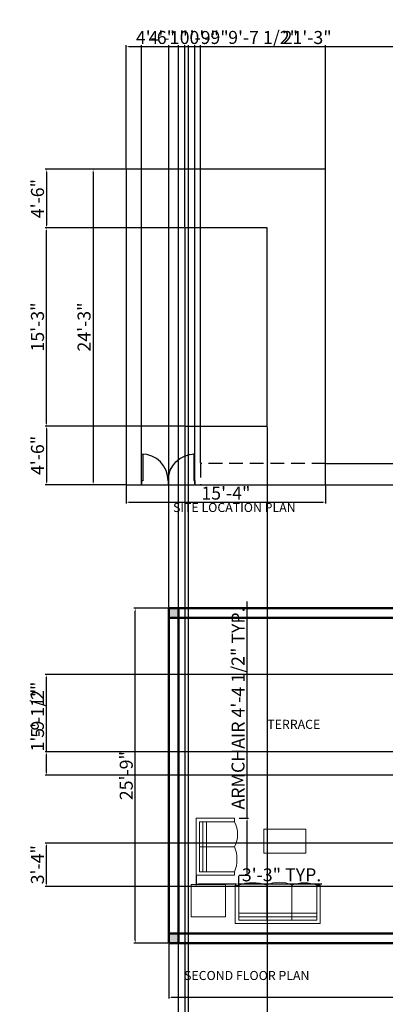
# Model space of a CAD drawing. Units: inches. Extents: x 1367 to 2309, y 1406 to 3826.
# Tile 7 of 9: x 1367 to 1704, y 2918 to 3826. Entities that reach past the tile are written whole.
import ezdxf

# ---------------------------------------------------------------- set-up
doc = ezdxf.new("R2010")
doc.units = ezdxf.units.IN
doc.linetypes.add('DASHED', pattern=[19.05, 12.7, -6.35])
for name, color, linetype, lineweight in [('A-ANNO-DIMS', 2, 'Continuous', 18), ('A-ANNO-TEXT', 7, 'Continuous', 25), ('A-AREA-IDEN', 3, 'Continuous', 18), ('A-DOOR', 4, 'Continuous', 25), ('A-FURN', 8, 'Continuous', 18), ('A-WALL', 7, 'Continuous', 50), ('A-WALL-PATT', 8, 'Continuous', 18), ('C-PROP', 7, 'Continuous', 25), ('C-PROP-LINE', 1, 'DASHED', 25)]:
    doc.layers.add(name, color=color, linetype=linetype, lineweight=lineweight)
doc.styles.get("Standard").update_dxf_attribs({"font": 'arial.ttf'})
doc.dimstyles.new('ISO-25', dxfattribs={"dimtxt": 12, "dimasz": 2.5, "dimexe": 1.25, "dimexo": 0.625, "dimtad": 1, "dimdec": 0, "dimlunit": 4, "dimtxsty": 'Standard', "dimcen": 2.5, "dimadec": 0, "dimazin": 0, "dimtfac": 1, "dimtdec": 0, "dimtmove": 0, "dimatfit": 3, "dimfxl": 1, "dimarcsym": 0})

# ---------------------------------------------------------------- blocks, each defined once
blk = doc.blocks.new('*U2')
for p, q in [((0, 0), (0, -6)), ((40, 0), (40, -6))]:
    blk.add_line(p, q)
blk.add_lwpolyline([(0, 0), (0, 40), (1.75, 40), (1.75, 0)], close=True)
blk.add_arc((0, 0), 40, 0, 90)
blk = doc.blocks.new('*D38')
at = {"layer": 'A-ANNO-DIMS', "color": 0, "lineweight": -2, "transparency": 16777216}
for p, q in [((1503.75, 3283.62), (1472.13, 3283.62)), ((1473.38, 2977.12), (1473.38, 3281.12)), ((1503.75, 2974.62), (1472.13, 2974.62))]:
    blk.add_line(p, q, dxfattribs=at)
at = {"layer": 'A-ANNO-DIMS', "color": 0, "lineweight": 100, "transparency": 16777216}
for points in [[(1472.96, 3281.12), (1473.79, 3281.12), (1473.38, 3283.62)], [(1472.96, 2977.12), (1473.79, 2977.12), (1473.38, 2974.62)]]:
    blk.add_solid(points, dxfattribs=at)
at = {"layer": 'Defpoints', "color": 0, "lineweight": 100, "transparency": 16777216}
for p in [(1473.38, 3283.62), (1504.37, 3283.62), (1504.37, 2974.62)]:
    blk.add_point(p, dxfattribs=at)
at = {"layer": 'A-ANNO-DIMS', "color": 0, "transparency": 16777216, "insert": (1466.62, 3129.12), "char_height": 12, "attachment_point": 5, "rotation": 90}
blk.add_mtext('25\'-9"', dxfattribs=at)
blk = doc.blocks.new('*D39')
at = {"layer": 'A-ANNO-DIMS', "color": 0, "lineweight": -2, "transparency": 16777216}
for p, q in [((1504.37, 2973.99), (1504.37, 2923.6)), ((2113.4, 2973.99), (2113.4, 2923.6)), ((1506.87, 2924.85), (2110.9, 2924.85))]:
    blk.add_line(p, q, dxfattribs=at)
at = {"layer": 'A-ANNO-DIMS', "color": 0, "lineweight": 100, "transparency": 16777216}
for points in [[(1506.87, 2925.27), (1506.87, 2924.44), (1504.37, 2924.85)], [(2110.9, 2925.27), (2110.9, 2924.44), (2113.4, 2924.85)]]:
    blk.add_solid(points, dxfattribs=at)
at = {"layer": 'Defpoints', "color": 0, "lineweight": 100, "transparency": 16777216}
for p in [(1504.37, 2974.62), (2113.4, 2974.62), (2113.4, 2924.85)]:
    blk.add_point(p, dxfattribs=at)
at = {"layer": 'A-ANNO-DIMS', "color": 0, "transparency": 16777216, "insert": (1808.89, 2931.6), "char_height": 12, "attachment_point": 5}
blk.add_mtext('50\'-9"', dxfattribs=at)
blk = doc.blocks.new('*D40')
at = {"layer": 'A-ANNO-DIMS', "color": 0, "lineweight": -2, "transparency": 16777216}
for p, q in [((1464.39, 3688.12), (1433.26, 3688.12)), ((1434.51, 3685.62), (1434.51, 3399.83)), ((1464.39, 3397.33), (1433.26, 3397.33))]:
    blk.add_line(p, q, dxfattribs=at)
at = {"layer": 'A-ANNO-DIMS', "color": 0, "lineweight": 100, "transparency": 16777216}
for points in [[(1434.09, 3685.62), (1434.92, 3685.62), (1434.51, 3688.12)], [(1434.09, 3399.83), (1434.92, 3399.83), (1434.51, 3397.33)]]:
    blk.add_solid(points, dxfattribs=at)
at = {"layer": 'Defpoints', "color": 0, "lineweight": 100, "transparency": 16777216}
for p in [(1465.02, 3688.12), (1434.51, 3397.33), (1465.02, 3397.33)]:
    blk.add_point(p, dxfattribs=at)
at = {"layer": 'A-ANNO-DIMS', "color": 0, "transparency": 16777216, "insert": (1427.75, 3542.73), "char_height": 12, "attachment_point": 5, "rotation": 90}
blk.add_mtext('24\'-3"', dxfattribs=at)
blk = doc.blocks.new('*D41')
at = {"layer": 'A-ANNO-DIMS', "color": 0, "lineweight": -2, "transparency": 16777216}
for p, q in [((1465.02, 3396.71), (1465.02, 3380.03)), ((1648.94, 3396.71), (1648.94, 3380.03)), ((1467.52, 3381.28), (1646.44, 3381.28))]:
    blk.add_line(p, q, dxfattribs=at)
at = {"layer": 'A-ANNO-DIMS', "color": 0, "lineweight": 100, "transparency": 16777216}
for points in [[(1467.52, 3381.7), (1467.52, 3380.86), (1465.02, 3381.28)], [(1646.44, 3381.7), (1646.44, 3380.86), (1648.94, 3381.28)]]:
    blk.add_solid(points, dxfattribs=at)
at = {"layer": 'Defpoints', "color": 0, "lineweight": 100, "transparency": 16777216}
for p in [(1465.02, 3397.33), (1648.94, 3397.33), (1648.94, 3381.28)]:
    blk.add_point(p, dxfattribs=at)
at = {"layer": 'A-ANNO-DIMS', "color": 0, "transparency": 16777216, "insert": (1556.98, 3388.03), "char_height": 12, "attachment_point": 5}
blk.add_mtext('15\'-4"', dxfattribs=at)
blk = doc.blocks.new('SOFA-3')
for p, q in [((3.39, 35.52), (0, 35.52)), ((0, 35.52), (0, 0)), ((29.28, 35.52), (29.28, 3.13)), ((52.37, 35.52), (52.37, 3.13)), ((75.45, 35.52), (78.61, 35.52)), ((78.61, 0), (78.61, 35.52)), ((0, 0), (78.61, 0))]:
    blk.add_line(p, q)
blk.add_lwpolyline([(3.39, 35.52), (3.39, 3.13), (75.45, 3.13), (75.45, 35.52)])
for centre, radius, start, end in [((16.33, -1.36), 39.09, 70.66096, 109.33904), ((40.82, 12.11), 26.1, 63.74962, 116.25038), ((63.91, 5.49), 32.17, 68.97185, 111.02815)]:
    blk.add_arc(centre, radius, start, end)
blk = doc.blocks.new('ARMCHAIR')
for p, q in [((0, 52.73), (0, 0)), ((35.52, 52.73), (0, 52.73)), ((35.52, 49.34), (3.13, 49.34)), ((35.52, 49.34), (35.52, 52.73)), ((35.52, 26.25), (3.13, 26.25)), ((35.52, 3.16), (35.52, 0)), ((0, 0), (35.52, 0))]:
    blk.add_line(p, q)
blk.add_lwpolyline([(3.13, 49.34), (3.13, 3.16), (35.52, 3.16)])
for centre, radius, start, end in [((12.11, 37.79), 26.1, 333.74962, 26.25038), ((5.49, 14.7), 32.17, 338.97185, 21.02815)]:
    blk.add_arc(centre, radius, start, end)
blk = doc.blocks.new('*D53')
at = {"layer": 'A-ANNO-DIMS', "color": 0, "lineweight": -2, "transparency": 16777216}
for p, q in [((1576.53, 3089.97), (1576.53, 3289.6)), ((1569.25, 3089.97), (1577.78, 3089.97)), ((1576.53, 3039.74), (1576.53, 3087.47)), ((1569.25, 3037.24), (1577.78, 3037.24))]:
    blk.add_line(p, q, dxfattribs=at)
at = {"layer": 'A-ANNO-DIMS', "color": 0, "lineweight": 100, "transparency": 16777216}
for points in [[(1576.11, 3087.47), (1576.95, 3087.47), (1576.53, 3089.97)], [(1576.11, 3039.74), (1576.95, 3039.74), (1576.53, 3037.24)]]:
    blk.add_solid(points, dxfattribs=at)
at = {"layer": 'Defpoints', "color": 0, "lineweight": 100, "transparency": 16777216}
for p in [(1568.62, 3089.97), (1576.53, 3089.97), (1568.62, 3037.24)]:
    blk.add_point(p, dxfattribs=at)
at = {"layer": 'A-ANNO-DIMS', "color": 0, "transparency": 16777216, "insert": (1569.7, 3191.04), "char_height": 12, "attachment_point": 5, "rotation": 90}
blk.add_mtext('ARMCHAIR 4\'-4 1/2" TYP.', dxfattribs=at)
blk = doc.blocks.new('*D54')
at = {"layer": 'A-ANNO-DIMS', "color": 0, "lineweight": -2, "transparency": 16777216}
for p, q in [((1529.51, 3036.62), (1529.51, 3028.08)), ((1568.62, 3036.62), (1568.62, 3028.08)), ((1532.01, 3029.33), (1566.12, 3029.33)), ((1568.62, 3029.33), (1645.51, 3029.33))]:
    blk.add_line(p, q, dxfattribs=at)
at = {"layer": 'A-ANNO-DIMS', "color": 0, "lineweight": 100, "transparency": 16777216}
for points in [[(1532.01, 3029.75), (1532.01, 3028.92), (1529.51, 3029.33)], [(1566.12, 3029.75), (1566.12, 3028.92), (1568.62, 3029.33)]]:
    blk.add_solid(points, dxfattribs=at)
at = {"layer": 'Defpoints', "color": 0, "lineweight": 100, "transparency": 16777216}
for p in [(1529.51, 3037.24), (1568.62, 3037.24), (1568.62, 3029.33)]:
    blk.add_point(p, dxfattribs=at)
at = {"layer": 'A-ANNO-DIMS', "color": 0, "transparency": 16777216, "insert": (1608.31, 3036.09), "char_height": 12, "attachment_point": 5}
blk.add_mtext('3\'-3" TYP.', dxfattribs=at)
blk = doc.blocks.new('*D87')
at = {"layer": 'A-ANNO-DIMS', "color": 0, "lineweight": -2, "transparency": 16777216}
for p, q in [((1513.37, 2814.79), (1513.37, 3802.6)), ((1515.87, 3801.35), (2110.9, 3801.35)), ((2113.4, 2814.79), (2113.4, 3802.6))]:
    blk.add_line(p, q, dxfattribs=at)
at = {"layer": 'A-ANNO-DIMS', "color": 0, "lineweight": 100, "transparency": 16777216}
for points in [[(1515.87, 3801.77), (1515.87, 3800.93), (1513.37, 3801.35)], [(2110.9, 3801.77), (2110.9, 3800.93), (2113.4, 3801.35)]]:
    blk.add_solid(points, dxfattribs=at)
at = {"layer": 'Defpoints', "color": 0, "lineweight": 100, "transparency": 16777216}
for p in [(2113.4, 3801.35), (1513.37, 2814.17), (2113.4, 2814.17)]:
    blk.add_point(p, dxfattribs=at)
at = {"layer": 'A-ANNO-DIMS', "color": 0, "transparency": 16777216, "insert": (1813.39, 3808.1), "char_height": 12, "attachment_point": 5}
blk.add_mtext('50\'-0"', dxfattribs=at)
blk = doc.blocks.new('*D88')
at = {"layer": 'A-ANNO-DIMS', "color": 0, "lineweight": -2, "transparency": 16777216}
for p, q in [((1513.37, 2814.79), (1513.37, 3802.6)), ((1515.87, 3801.35), (1519.87, 3801.35)), ((1522.37, 2805.79), (1522.37, 3802.6)), ((1522.37, 3801.35), (1558.02, 3801.35))]:
    blk.add_line(p, q, dxfattribs=at)
at = {"layer": 'A-ANNO-DIMS', "color": 0, "lineweight": 100, "transparency": 16777216}
for points in [[(1515.87, 3801.77), (1515.87, 3800.93), (1513.37, 3801.35)], [(1519.87, 3801.77), (1519.87, 3800.93), (1522.37, 3801.35)]]:
    blk.add_solid(points, dxfattribs=at)
at = {"layer": 'Defpoints', "color": 0, "lineweight": 100, "transparency": 16777216}
for p in [(1522.37, 3801.35), (1513.37, 2814.17), (1522.37, 2805.17)]:
    blk.add_point(p, dxfattribs=at)
at = {"layer": 'A-ANNO-DIMS', "color": 0, "transparency": 16777216, "insert": (1541.44, 3808.1), "char_height": 12, "attachment_point": 5}
blk.add_mtext('0\'-9"', dxfattribs=at)
blk = doc.blocks.new('*D103')
at = {"layer": 'A-ANNO-DIMS', "color": 0, "lineweight": -2, "transparency": 16777216}
for p, q in [((1504.37, 3284.24), (1504.37, 3802.6)), ((1506.87, 3801.35), (1756.92, 3801.35)), ((1759.42, 3284.24), (1759.42, 3802.6))]:
    blk.add_line(p, q, dxfattribs=at)
at = {"layer": 'A-ANNO-DIMS', "color": 0, "lineweight": 100, "transparency": 16777216}
for points in [[(1506.87, 3801.77), (1506.87, 3800.93), (1504.37, 3801.35)], [(1756.92, 3801.77), (1756.92, 3800.93), (1759.42, 3801.35)]]:
    blk.add_solid(points, dxfattribs=at)
at = {"layer": 'Defpoints', "color": 0, "lineweight": 100, "transparency": 16777216}
for p in [(1759.42, 3801.35), (1504.37, 3283.62), (1759.42, 3283.62)]:
    blk.add_point(p, dxfattribs=at)
at = {"layer": 'A-ANNO-DIMS', "color": 0, "transparency": 16777216, "insert": (1631.89, 3808.1), "char_height": 12, "attachment_point": 5}
blk.add_mtext('21\'-3"', dxfattribs=at)
blk = doc.blocks.new('*D104')
at = {"layer": 'A-ANNO-DIMS', "color": 0, "lineweight": -2, "transparency": 16777216}
for p, q in [((1504.37, 3284.24), (1504.37, 3802.6)), ((1506.87, 3801.35), (1510.87, 3801.35)), ((1513.37, 3275.24), (1513.37, 3802.6)), ((1513.37, 3801.35), (1549.02, 3801.35))]:
    blk.add_line(p, q, dxfattribs=at)
at = {"layer": 'A-ANNO-DIMS', "color": 0, "lineweight": 100, "transparency": 16777216}
for points in [[(1506.87, 3801.77), (1506.87, 3800.93), (1504.37, 3801.35)], [(1510.87, 3801.77), (1510.87, 3800.93), (1513.37, 3801.35)]]:
    blk.add_solid(points, dxfattribs=at)
at = {"layer": 'Defpoints', "color": 0, "lineweight": 100, "transparency": 16777216}
for p in [(1513.37, 3801.35), (1504.37, 3283.62), (1513.37, 3274.62)]:
    blk.add_point(p, dxfattribs=at)
at = {"layer": 'A-ANNO-DIMS', "color": 0, "transparency": 16777216, "insert": (1532.44, 3808.1), "char_height": 12, "attachment_point": 5}
blk.add_mtext('0\'-9"', dxfattribs=at)
blk = doc.blocks.new('*D109')
at = {"layer": 'A-ANNO-DIMS', "color": 0, "lineweight": -2, "transparency": 16777216}
for p, q in [((1963.5, 3066.97), (1390.27, 3066.97)), ((1391.52, 3029.47), (1391.52, 3064.47)), ((1963.5, 3026.97), (1390.27, 3026.97))]:
    blk.add_line(p, q, dxfattribs=at)
at = {"layer": 'A-ANNO-DIMS', "color": 0, "lineweight": 100, "transparency": 16777216}
for points in [[(1391.1, 3064.47), (1391.94, 3064.47), (1391.52, 3066.97)], [(1391.1, 3029.47), (1391.94, 3029.47), (1391.52, 3026.97)]]:
    blk.add_solid(points, dxfattribs=at)
at = {"layer": 'Defpoints', "color": 0, "lineweight": 100, "transparency": 16777216}
for p in [(1391.52, 3066.97), (1964.13, 3066.97), (1964.13, 3026.97)]:
    blk.add_point(p, dxfattribs=at)
at = {"layer": 'A-ANNO-DIMS', "color": 0, "transparency": 16777216, "insert": (1384.76, 3046.97), "char_height": 12, "attachment_point": 5, "rotation": 90}
blk.add_mtext('3\'-4"', dxfattribs=at)
blk = doc.blocks.new('*D124')
at = {"layer": 'A-ANNO-DIMS', "color": 0, "lineweight": -2, "transparency": 16777216}
for p, q in [((1391.52, 3151.06), (1391.52, 3213.55)), ((1819.79, 3151.06), (1390.27, 3151.06)), ((1391.52, 3132.02), (1391.52, 3148.56)), ((1819.79, 3129.52), (1390.27, 3129.52))]:
    blk.add_line(p, q, dxfattribs=at)
at = {"layer": 'A-ANNO-DIMS', "color": 0, "lineweight": 100, "transparency": 16777216}
for points in [[(1391.1, 3148.56), (1391.94, 3148.56), (1391.52, 3151.06)], [(1391.1, 3132.02), (1391.94, 3132.02), (1391.52, 3129.52)]]:
    blk.add_solid(points, dxfattribs=at)
at = {"layer": 'Defpoints', "color": 0, "lineweight": 100, "transparency": 16777216}
for p in [(1391.52, 3151.06), (1820.42, 3151.06), (1820.42, 3129.52)]:
    blk.add_point(p, dxfattribs=at)
at = {"layer": 'A-ANNO-DIMS', "color": 0, "transparency": 16777216, "insert": (1384.69, 3183.56), "char_height": 12, "attachment_point": 5, "rotation": 90}
blk.add_mtext('1\'-9 1/2"', dxfattribs=at)
blk = doc.blocks.new('*D126')
at = {"layer": 'A-ANNO-DIMS', "color": 0, "lineweight": -2, "transparency": 16777216}
for p, q in [((1975.08, 3222.26), (1390.27, 3222.26)), ((1391.52, 3153.56), (1391.52, 3219.76)), ((1975.08, 3151.06), (1390.27, 3151.06))]:
    blk.add_line(p, q, dxfattribs=at)
at = {"layer": 'A-ANNO-DIMS', "color": 0, "lineweight": 100, "transparency": 16777216}
for points in [[(1391.1, 3219.76), (1391.94, 3219.76), (1391.52, 3222.26)], [(1391.1, 3153.56), (1391.94, 3153.56), (1391.52, 3151.06)]]:
    blk.add_solid(points, dxfattribs=at)
at = {"layer": 'Defpoints', "color": 0, "lineweight": 100, "transparency": 16777216}
for p in [(1391.52, 3222.26), (1975.7, 3222.26), (1975.7, 3151.06)]:
    blk.add_point(p, dxfattribs=at)
at = {"layer": 'A-ANNO-DIMS', "color": 0, "transparency": 16777216, "insert": (1384.77, 3186.66), "char_height": 12, "attachment_point": 5, "rotation": 90}
blk.add_mtext('5\'-11"', dxfattribs=at)
blk = doc.blocks.new('*D127')
at = {"layer": 'A-ANNO-DIMS', "color": 0, "lineweight": -2, "transparency": 16777216}
for p, q in [((1519.02, 3450.71), (1519.02, 2257.28)), ((1594.94, 3450.71), (1594.94, 2257.28)), ((1521.52, 2258.53), (1592.44, 2258.53))]:
    blk.add_line(p, q, dxfattribs=at)
at = {"layer": 'A-ANNO-DIMS', "color": 0, "lineweight": 100, "transparency": 16777216}
for points in [[(1521.52, 2258.94), (1521.52, 2258.11), (1519.02, 2258.53)], [(1592.44, 2258.94), (1592.44, 2258.11), (1594.94, 2258.53)]]:
    blk.add_solid(points, dxfattribs=at)
at = {"layer": 'Defpoints', "color": 0, "lineweight": 100, "transparency": 16777216}
for p in [(1519.02, 3451.33), (1594.94, 3451.33), (1594.94, 2258.53)]:
    blk.add_point(p, dxfattribs=at)
at = {"layer": 'A-ANNO-DIMS', "color": 0, "transparency": 16777216, "insert": (1556.98, 2265.28), "char_height": 12, "attachment_point": 5}
blk.add_mtext('6\'-4"', dxfattribs=at)
blk = doc.blocks.new('*D128')
at = {"layer": 'A-ANNO-DIMS', "color": 0, "lineweight": -2, "transparency": 16777216}
for p, q in [((1518.39, 3634.12), (1390.27, 3634.12)), ((1391.52, 3453.83), (1391.52, 3631.62)), ((1518.39, 3451.33), (1390.27, 3451.33))]:
    blk.add_line(p, q, dxfattribs=at)
at = {"layer": 'A-ANNO-DIMS', "color": 0, "lineweight": 100, "transparency": 16777216}
for points in [[(1391.1, 3631.62), (1391.94, 3631.62), (1391.52, 3634.12)], [(1391.1, 3453.83), (1391.94, 3453.83), (1391.52, 3451.33)]]:
    blk.add_solid(points, dxfattribs=at)
at = {"layer": 'Defpoints', "color": 0, "lineweight": 100, "transparency": 16777216}
for p in [(1391.52, 3634.12), (1519.02, 3634.12), (1519.02, 3451.33)]:
    blk.add_point(p, dxfattribs=at)
at = {"layer": 'A-ANNO-DIMS', "color": 0, "transparency": 16777216, "insert": (1384.76, 3542.73), "char_height": 12, "attachment_point": 5, "rotation": 90}
blk.add_mtext('15\'-3"', dxfattribs=at)
blk = doc.blocks.new('*D129')
at = {"layer": 'A-ANNO-DIMS', "color": 0, "lineweight": -2, "transparency": 16777216}
for p, q in [((1465.02, 3688.74), (1465.02, 3802.6)), ((1467.52, 3801.35), (1516.52, 3801.35)), ((1519.02, 3634.74), (1519.02, 3802.6))]:
    blk.add_line(p, q, dxfattribs=at)
at = {"layer": 'A-ANNO-DIMS', "color": 0, "lineweight": 100, "transparency": 16777216}
for points in [[(1467.52, 3801.77), (1467.52, 3800.93), (1465.02, 3801.35)], [(1516.52, 3801.77), (1516.52, 3800.93), (1519.02, 3801.35)]]:
    blk.add_solid(points, dxfattribs=at)
at = {"layer": 'Defpoints', "color": 0, "lineweight": 100, "transparency": 16777216}
for p in [(1519.02, 3801.35), (1465.02, 3688.12), (1519.02, 3634.12)]:
    blk.add_point(p, dxfattribs=at)
at = {"layer": 'A-ANNO-DIMS', "color": 0, "transparency": 16777216, "insert": (1492.02, 3808.1), "char_height": 12, "attachment_point": 5}
blk.add_mtext('4\'-6"', dxfattribs=at)
blk = doc.blocks.new('*D130')
at = {"layer": 'A-ANNO-DIMS', "color": 0, "lineweight": -2, "transparency": 16777216}
for p, q in [((1464.39, 3688.12), (1390.27, 3688.12)), ((1391.52, 3685.62), (1391.52, 3636.62)), ((1518.39, 3634.12), (1390.27, 3634.12))]:
    blk.add_line(p, q, dxfattribs=at)
at = {"layer": 'A-ANNO-DIMS', "color": 0, "lineweight": 100, "transparency": 16777216}
for points in [[(1391.1, 3685.62), (1391.94, 3685.62), (1391.52, 3688.12)], [(1391.1, 3636.62), (1391.94, 3636.62), (1391.52, 3634.12)]]:
    blk.add_solid(points, dxfattribs=at)
at = {"layer": 'Defpoints', "color": 0, "lineweight": 100, "transparency": 16777216}
for p in [(1465.02, 3688.12), (1391.52, 3634.12), (1519.02, 3634.12)]:
    blk.add_point(p, dxfattribs=at)
at = {"layer": 'A-ANNO-DIMS', "color": 0, "transparency": 16777216, "insert": (1384.77, 3661.12), "char_height": 12, "attachment_point": 5, "rotation": 90}
blk.add_mtext('4\'-6"', dxfattribs=at)
blk = doc.blocks.new('*D131')
at = {"layer": 'A-ANNO-DIMS', "color": 0, "lineweight": -2, "transparency": 16777216}
for p, q in [((1518.39, 3451.33), (1390.27, 3451.33)), ((1391.52, 3448.83), (1391.52, 3399.83)), ((1464.39, 3397.33), (1390.27, 3397.33))]:
    blk.add_line(p, q, dxfattribs=at)
at = {"layer": 'A-ANNO-DIMS', "color": 0, "lineweight": 100, "transparency": 16777216}
for points in [[(1391.1, 3448.83), (1391.94, 3448.83), (1391.52, 3451.33)], [(1391.1, 3399.83), (1391.94, 3399.83), (1391.52, 3397.33)]]:
    blk.add_solid(points, dxfattribs=at)
at = {"layer": 'Defpoints', "color": 0, "lineweight": 100, "transparency": 16777216}
for p in [(1519.02, 3451.33), (1391.52, 3397.33), (1465.02, 3397.33)]:
    blk.add_point(p, dxfattribs=at)
at = {"layer": 'A-ANNO-DIMS', "color": 0, "transparency": 16777216, "insert": (1384.77, 3424.33), "char_height": 12, "attachment_point": 5, "rotation": 90}
blk.add_mtext('4\'-6"', dxfattribs=at)
blk = doc.blocks.new('*D132')
at = {"layer": 'A-ANNO-DIMS', "color": 0, "lineweight": -2, "transparency": 16777216}
for p, q in [((1479.16, 3397.96), (1479.16, 3802.6)), ((1481.66, 3801.35), (1525.83, 3801.35)), ((1528.33, 3398.02), (1528.33, 3802.6))]:
    blk.add_line(p, q, dxfattribs=at)
at = {"layer": 'A-ANNO-DIMS', "color": 0, "lineweight": 100, "transparency": 16777216}
for points in [[(1481.66, 3801.77), (1481.66, 3800.93), (1479.16, 3801.35)], [(1525.83, 3801.77), (1525.83, 3800.93), (1528.33, 3801.35)]]:
    blk.add_solid(points, dxfattribs=at)
at = {"layer": 'Defpoints', "color": 0, "lineweight": 100, "transparency": 16777216}
for p in [(1528.33, 3801.35), (1479.16, 3397.33), (1528.33, 3397.4)]:
    blk.add_point(p, dxfattribs=at)
at = {"layer": 'A-ANNO-DIMS', "color": 0, "transparency": 16777216, "insert": (1503.74, 3808), "char_height": 12, "attachment_point": 5}
blk.add_mtext('4\'-1"', dxfattribs=at)
blk = doc.blocks.new('*D133')
at = {"layer": 'A-ANNO-DIMS', "color": 0, "lineweight": -2, "transparency": 16777216}
for p, q in [((1533.64, 3417.41), (1533.64, 3802.6)), ((1536.14, 3801.35), (1646.44, 3801.35)), ((1648.94, 3417.41), (1648.94, 3802.6))]:
    blk.add_line(p, q, dxfattribs=at)
at = {"layer": 'A-ANNO-DIMS', "color": 0, "lineweight": 100, "transparency": 16777216}
for points in [[(1536.14, 3801.77), (1536.14, 3800.93), (1533.64, 3801.35)], [(1646.44, 3801.77), (1646.44, 3800.93), (1648.94, 3801.35)]]:
    blk.add_solid(points, dxfattribs=at)
at = {"layer": 'Defpoints', "color": 0, "lineweight": 100, "transparency": 16777216}
for p in [(1648.94, 3801.35), (1533.64, 3416.79), (1648.94, 3416.79)]:
    blk.add_point(p, dxfattribs=at)
at = {"layer": 'A-ANNO-DIMS', "color": 0, "transparency": 16777216, "insert": (1591.29, 3808.18), "char_height": 12, "attachment_point": 5}
blk.add_mtext('9\'-7 1/2"', dxfattribs=at)
blk = doc.blocks.new('*D134')
at = {"layer": 'A-ANNO-DIMS', "color": 0, "lineweight": -2, "transparency": 16777216}
for p, q in [((2298.26, 3416.79), (2298.26, 3479.27)), ((1649.56, 3416.79), (2299.51, 3416.79)), ((2298.26, 3399.83), (2298.26, 3414.29)), ((1649.56, 3397.33), (2299.51, 3397.33))]:
    blk.add_line(p, q, dxfattribs=at)
at = {"layer": 'A-ANNO-DIMS', "color": 0, "lineweight": 100, "transparency": 16777216}
for points in [[(2297.84, 3414.29), (2298.67, 3414.29), (2298.26, 3416.79)], [(2297.84, 3399.83), (2298.67, 3399.83), (2298.26, 3397.33)]]:
    blk.add_solid(points, dxfattribs=at)
at = {"layer": 'Defpoints', "color": 0, "lineweight": 100, "transparency": 16777216}
for p in [(1648.94, 3416.79), (2298.26, 3416.79), (1648.94, 3397.33)]:
    blk.add_point(p, dxfattribs=at)
at = {"layer": 'A-ANNO-DIMS', "color": 0, "transparency": 16777216, "insert": (2291.43, 3449.28), "char_height": 12, "attachment_point": 5, "rotation": 90}
blk.add_mtext('1\'-7 1/2"', dxfattribs=at)

msp = doc.modelspace()

# ---------------------------------------------------------------- hatches: boundary and pattern name
at = {"layer": 'A-WALL-PATT'}
h = msp.add_hatch(color=256, dxfattribs=at)
h.dxf.hatch_style = 1
h.paths.add_polyline_path([(1513.37, 2983.62), (1504.37, 2983.62), (1504.37, 2974.62), (1513.37, 2974.62)])
h.paths.add_polyline_path([(1759.42, 2983.62), (1749.82, 2983.62), (1749.82, 2974.62), (1759.42, 2974.62)])
h.paths.add_polyline_path([(1513.37, 3283.62), (1504.37, 3283.62), (1504.37, 3274.62), (1513.37, 3274.62)])
h.paths.add_polyline_path([(1759.42, 3283.62), (1750.75, 3283.62), (1750.75, 3274.62), (1759.42, 3274.62)])
h.paths.add_polyline_path([(2113.4, 2983.62), (2104.4, 2983.62), (2104.4, 2974.62), (2113.4, 2974.62)])
h.paths.add_polyline_path([(1787.87, 2343.17), (1778.87, 2343.17), (1778.87, 2334.17), (1787.87, 2334.17)])
h.paths.add_polyline_path([(1964.87, 2343.17), (1960.37, 2343.17), (1955.87, 2343.17), (1955.87, 2334.17), (1964.87, 2334.17)])
h.paths.add_polyline_path([(2113.37, 2343.17), (2104.37, 2343.17), (2104.37, 2334.17), (2113.37, 2334.17)])
h.paths.add_polyline_path([(1783.37, 2513.73), (1774.44, 2513.73), (1774.44, 2504.73), (1783.37, 2504.73)])
h.paths.add_polyline_path([(1787.54, 2814.17), (1778.54, 2814.17), (1778.54, 2805.17), (1787.54, 2805.17)])
h.paths.add_polyline_path([(1964.87, 2814.17), (1955.87, 2814.17), (1955.87, 2805.17), (1964.87, 2805.17)])
h.paths.add_polyline_path([(2113.37, 2814.17), (2104.4, 2814.17), (2104.4, 2805.17), (2113.37, 2805.17)])
h.paths.add_polyline_path([(1522.37, 2814.17), (1513.37, 2814.17), (1513.37, 2805.17), (1522.37, 2805.17)])
h.paths.add_polyline_path([(2019.97, 2440.35), (2070.2, 2440.35), (2070.2, 2457.56), (2019.97, 2457.56)], flags=9)
h.paths.add_polyline_path([(1670.17, 2422.1), (1711.32, 2422.1), (1711.32, 2439.31), (1670.17, 2439.31)], flags=9)
h.paths.add_polyline_path([(1917.64, 2783.38), (1946.46, 2783.38), (1946.46, 2800.59), (1917.64, 2800.59)], flags=9)
h.paths.add_polyline_path([(1526.17, 2423.16), (1570.57, 2423.16), (1570.57, 2440.37), (1526.17, 2440.37)], flags=9)
h.paths.add_polyline_path([(2013.98, 2676.57), (2064.21, 2676.57), (2064.21, 2693.79), (2013.98, 2693.79)], flags=9)
h.paths.add_polyline_path([(1738.47, 2785.04), (1767.29, 2785.04), (1767.29, 2802.25), (1738.47, 2802.25)], flags=9)
h.paths.add_polyline_path([(1832.32, 2473.89), (1889.69, 2473.89), (1889.69, 2491.1), (1832.32, 2491.1)], flags=9)
h.paths.add_polyline_path([(1821.9, 2712.75), (1863.05, 2712.75), (1863.05, 2729.96), (1821.9, 2729.96)], flags=9)
h.paths.add_polyline_path([(1595.64, 2683.62), (1684.77, 2683.62), (1684.77, 2700.83), (1595.64, 2700.83)], flags=9)

# ---------------------------------------------------------------- linework, layer by layer
at = {"layer": 'A-FURN'}
for p, q in [((1535.84, 3086.58), (1535.84, 3040.4)), ((1539.19, 3086.58), (1539.19, 3040.4)), ((1568.79, 3002.37), (1640.85, 3002.37)), ((1568.79, 2999.02), (1640.85, 2999.02))]:
    msp.add_line(p, q, dxfattribs=at)
for points in [[(1591.88, 3079.82), (1630.69, 3079.82), (1630.69, 3057.49), (1591.88, 3057.49)], [(1524.94, 2998.85), (1556.66, 2998.85), (1556.66, 3028.67), (1524.94, 3028.67)]]:
    msp.add_lwpolyline(points, close=True, dxfattribs=at)
at = {"layer": 'A-WALL'}
for p, q in [((1504.37, 3283.62), (1759.42, 3283.62)), ((1504.37, 2974.62), (1504.37, 3283.62)), ((1513.37, 2983.62), (1513.37, 3274.62)), ((1513.37, 3274.62), (1754.92, 3274.62)), ((1754.92, 2983.62), (1513.37, 2983.62)), ((1504.37, 2974.62), (2113.4, 2974.62))]:
    msp.add_line(p, q, dxfattribs=at)
for points in [[(1504.37, 3283.62), (1513.37, 3283.62), (1513.37, 3274.62), (1504.37, 3274.62)], [(1504.37, 2974.62), (1513.37, 2974.62), (1513.37, 2983.62), (1504.37, 2983.62)]]:
    msp.add_lwpolyline(points, close=True, dxfattribs=at)
at = {"layer": 'C-PROP'}
for points in [[(1465.02, 3397.33), (1648.94, 3397.33), (1648.94, 3688.12), (1465.02, 3688.12)], [(1519.02, 3451.33), (1594.94, 3451.33), (1594.94, 3634.12), (1519.02, 3634.12)]]:
    msp.add_lwpolyline(points, close=True, dxfattribs=at)
at = {"layer": 'C-PROP-LINE'}
msp.add_lwpolyline([(1533.64, 3397.33), (1648.94, 3397.33), (1648.94, 3416.79), (1533.64, 3416.79)], close=True, dxfattribs=at)

# ---------------------------------------------------------------- block references
at = {"layer": 'A-DOOR', "yscale": 0.6146277192172834, "zscale": 0.6146277192172834}
for p, xscale in [((1479.16, 3401.02), 0.6146277192172834), ((1528.33, 3401.08), -0.6146277192172834)]:
    msp.add_blockref('*U2', p, dxfattribs=dict(at, xscale=xscale))
at = {"layer": 'A-FURN'}
for name, p in [('ARMCHAIR', (1529.51, 3037.24)), ('SOFA-3', (1565.4, 2992.69))]:
    msp.add_blockref(name, p, dxfattribs=at)

# ---------------------------------------------------------------- texts
at = {"layer": 'A-ANNO-TEXT', "char_height": 8.3529, "attachment_point": 1}
for s, insert in [('SITE LOCATION PLAN', (1508.24, 3380.52)), ('SECOND FLOOR PLAN', (1518.39, 2949.02))]:
    msp.add_mtext_dynamic_manual_height_columns(s, width=204.251, gutter_width=41.76, heights=[0], dxfattribs=dict(at, insert=insert))
at = {"layer": 'A-AREA-IDEN', "insert": (1595.12, 3180.59), "char_height": 8.353, "attachment_point": 1}
msp.add_mtext_dynamic_manual_height_columns('TERRACE', width=204.251, gutter_width=41.76, heights=[0], dxfattribs=at)

# ---------------------------------------------------------------- dimensions: what is measured, and where the dimension line sits
at = {"layer": 'A-ANNO-DIMS'}
for base, p1, p2, override, picture, middle in [((1648.94, 3801.35), (1533.64, 3416.79), (1648.94, 3416.79), {"dimdec": 1, "dimlfac": 1, "dimrnd": 0, "dimzin": 1, "dimdsep": 46, "dimlunit": 4, "dimfrac": 2}, '*D133', (1591.29, 3808.18)), ((1519.02, 3801.35), (1465.02, 3688.12), (1519.02, 3634.12), {"dimdec": 1, "dimlfac": 1, "dimrnd": 0, "dimzin": 1, "dimdsep": 46, "dimlunit": 4, "dimfrac": 2}, '*D129', (1492.02, 3808.1)), ((1528.33, 3801.35), (1479.16, 3397.33), (1528.33, 3397.4), {"dimdec": 1, "dimlfac": 1, "dimrnd": 0, "dimzin": 1, "dimdsep": 46, "dimlunit": 4, "dimfrac": 2}, '*D132', (1503.74, 3808)), ((1759.4169, 3801.349), (1504.3701, 3283.618), (1759.4169, 3283.618), {"dimdec": 1, "dimlfac": 1, "dimrnd": 0, "dimzin": 1, "dimdsep": 46, "dimlunit": 4, "dimfrac": 2}, '*D103', (1631.8935, 3808.105)), ((1513.37, 3801.35), (1504.37, 3283.62), (1513.37, 3274.62), {"dimdec": 1, "dimlfac": 1, "dimrnd": 0, "dimzin": 1, "dimdsep": 46, "dimlunit": 4, "dimfrac": 2}, '*D104', (1532.44, 3808.1)), ((2113.4, 3801.35), (1513.37, 2814.17), (2113.4, 2814.17), {"dimdec": 1, "dimlfac": 1, "dimrnd": 0, "dimzin": 1, "dimdsep": 46, "dimlunit": 4, "dimfrac": 2}, '*D87', (1813.39, 3808.1)), ((1522.37, 3801.35), (1513.37, 2814.17), (1522.37, 2805.17), {"dimdec": 1, "dimlfac": 1, "dimrnd": 0, "dimzin": 1, "dimdsep": 46, "dimlunit": 4, "dimfrac": 2}, '*D88', (1541.44, 3808.1)), ((1594.94, 2258.53), (1519.02, 3451.33), (1594.94, 3451.33), {"dimdec": 1, "dimlfac": 1, "dimrnd": 0, "dimzin": 1, "dimdsep": 46, "dimlunit": 4, "dimfrac": 2}, '*D127', (1556.98, 2265.28)), ((1648.94, 3381.28), (1465.02, 3397.33), (1648.94, 3397.33), {"dimclrd": 0, "dimclre": 0, "dimclrt": 0}, '*D41', (1556.98, 3388.03)), ((2113.4, 2924.85), (1504.37, 2974.62), (2113.4, 2974.62), {"dimclrd": 0, "dimclre": 0, "dimclrt": 0}, '*D39', (1808.89, 2931.6))]:
    dim = msp.add_linear_dim(base=base, p1=p1, p2=p2, dimstyle='ISO-25', override=override, dxfattribs=at)
    dim.commit()
    dim.dimension.update_dxf_attribs({"geometry": picture, "text_midpoint": middle})
for base, p1, p2, override, picture, middle in [((1391.52, 3634.12), (1465.02, 3688.12), (1519.02, 3634.12), {"dimdec": 1, "dimlfac": 1, "dimrnd": 0, "dimzin": 1, "dimdsep": 46, "dimlunit": 4, "dimfrac": 2}, '*D130', (1384.77, 3661.12)), ((1434.51, 3397.33), (1465.02, 3688.12), (1465.02, 3397.33), {"dimclrd": 0, "dimclre": 0, "dimclrt": 0}, '*D40', (1427.75, 3542.73)), ((1391.52, 3634.12), (1519.02, 3451.33), (1519.02, 3634.12), {"dimdec": 1, "dimlfac": 1, "dimrnd": 0, "dimzin": 1, "dimdsep": 46, "dimlunit": 4, "dimfrac": 2}, '*D128', (1384.76, 3542.73)), ((2298.26, 3416.79), (1648.94, 3397.33), (1648.94, 3416.79), {"dimdec": 1, "dimlfac": 1, "dimrnd": 0, "dimzin": 1, "dimdsep": 46, "dimlunit": 4, "dimfrac": 2}, '*D134', (2291.43, 3449.28)), ((1391.52, 3397.33), (1519.02, 3451.33), (1465.02, 3397.33), {"dimdec": 1, "dimlfac": 1, "dimrnd": 0, "dimzin": 1, "dimdsep": 46, "dimlunit": 4, "dimfrac": 2}, '*D131', (1384.77, 3424.33)), ((1473.38, 3283.62), (1504.37, 2974.62), (1504.37, 3283.62), {"dimclrd": 0, "dimclre": 0, "dimclrt": 0}, '*D38', (1466.62, 3129.12)), ((1391.52, 3151.06), (1820.42, 3129.52), (1820.42, 3151.06), {"dimdec": 1, "dimlfac": 1, "dimrnd": 0, "dimzin": 1, "dimdsep": 46, "dimlunit": 4, "dimfrac": 2}, '*D124', (1384.69, 3183.56)), ((1391.52, 3222.26), (1975.7, 3151.06), (1975.7, 3222.26), {"dimdec": 1, "dimlfac": 1, "dimrnd": 0, "dimzin": 1, "dimdsep": 46, "dimlunit": 4, "dimfrac": 2}, '*D126', (1384.77, 3186.66)), ((1391.52, 3066.97), (1964.13, 3026.97), (1964.13, 3066.97), {"dimdec": 1, "dimlfac": 1, "dimrnd": 0, "dimzin": 1, "dimdsep": 46, "dimlunit": 4, "dimfrac": 2}, '*D109', (1384.76, 3046.97))]:
    dim = msp.add_linear_dim(base=base, p1=p1, p2=p2, angle=90, dimstyle='ISO-25', override=override, dxfattribs=at)
    dim.commit()
    dim.dimension.update_dxf_attribs({"geometry": picture, "text_midpoint": middle})
dim = msp.add_linear_dim(base=(1576.53, 3089.97), p1=(1568.62, 3037.24), p2=(1568.62, 3089.97), angle=90, text='ARMCHAIR <> TYP.', dimstyle='ISO-25', override={"dimdec": 1, "dimrnd": 0, "dimzin": 1, "dimlunit": 4, "dimfrac": 2}, dxfattribs=at)
dim.commit()
dim.dimension.update_dxf_attribs({"geometry": '*D53', "text_midpoint": (1569.7, 3191.04)})
dim = msp.add_linear_dim(base=(1568.62, 3029.33), p1=(1529.51, 3037.24), p2=(1568.62, 3037.24), text='<> TYP.', dimstyle='ISO-25', override={"dimdec": 1, "dimrnd": 0, "dimzin": 1, "dimlunit": 4, "dimfrac": 2}, dxfattribs=at)
dim.commit()
dim.dimension.update_dxf_attribs({"geometry": '*D54', "text_midpoint": (1608.31, 3036.09)})

doc.saveas('drawing.dxf')
